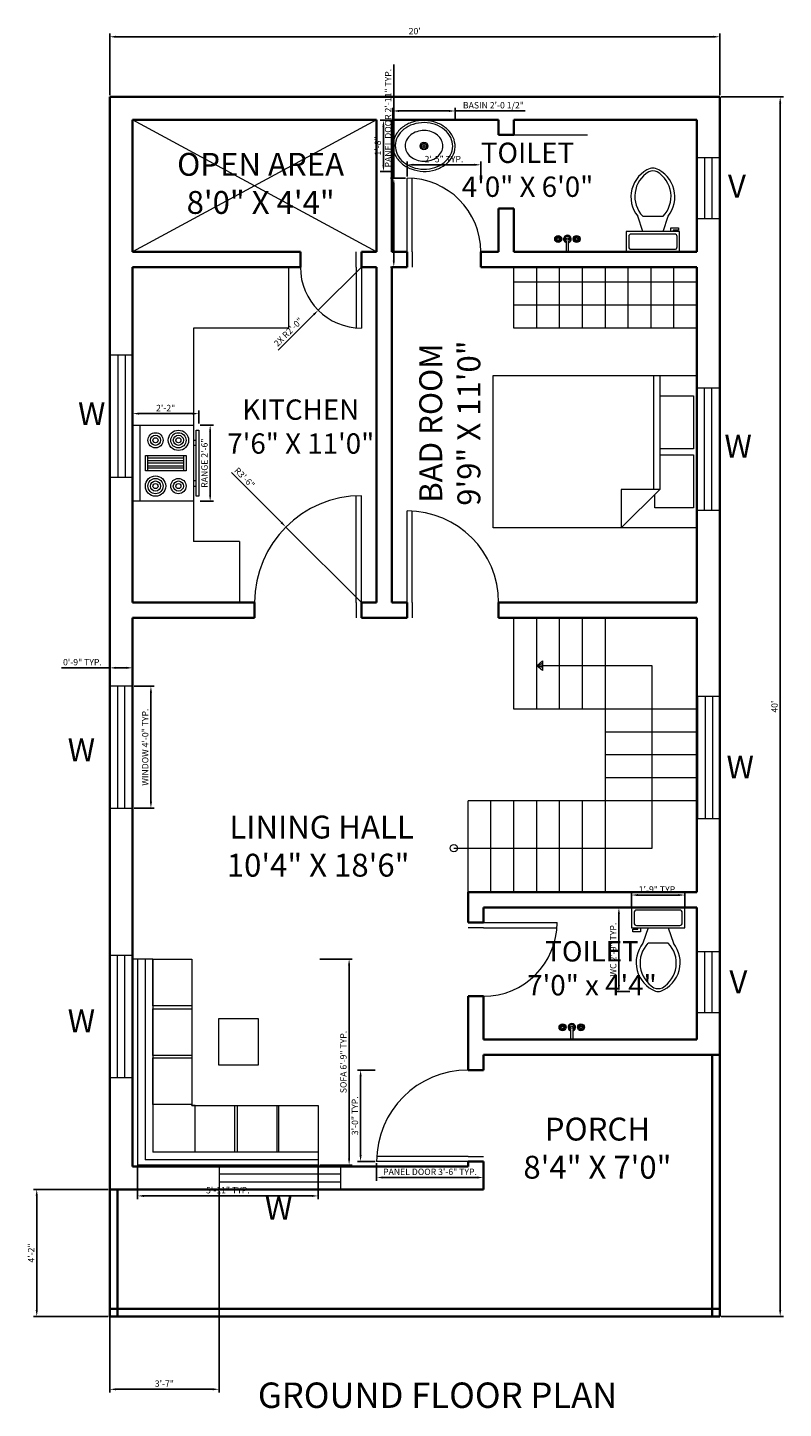
# Model space of a CAD drawing. Units: inches. Extents: x 1827 to 2455, y 1682 to 2281.
# Tile 1 of 3: x 1827 to 2124, y 1686 to 2229. Entities that reach past the tile are written whole.
import ezdxf

# ---------------------------------------------------------------- set-up
doc = ezdxf.new("R2010")
doc.units = ezdxf.units.IN
for name, color, linetype, lineweight in [('A-ANNO-DIMS', 2, 'Continuous', 18), ('A-ANNO-TEXT', 7, 'Continuous', 18), ('A-AREA-IDEN', 7, 'Continuous', 18), ('A-DOOR', 3, 'Continuous', 18), ('A-EQPM', 9, 'Continuous', 18), ('A-FLOR-CABN', 9, 'Continuous', 18), ('A-FLOR-FIXT', 9, 'Continuous', 18), ('A-FLOR-OPEN', 8, 'Continuous', 13), ('A-FLOR-STRS', 7, 'Continuous', 20), ('A-FURN', 8, 'Continuous', 18), ('A-GLAZ', 4, 'Continuous', 18), ('A-WALL', 7, 'Continuous', 35)]:
    doc.layers.add(name, color=color, linetype=linetype, lineweight=lineweight)
doc.styles.get("Standard").update_dxf_attribs({"font": 'arial.ttf'})
doc.dimstyles.new('ISO-25', dxfattribs={"dimtxt": 2.5, "dimasz": 2.5, "dimexe": 1.25, "dimexo": 0.625, "dimtad": 1, "dimdec": 0, "dimlunit": 3, "dimtxsty": 'Standard', "dimcen": 2.5, "dimadec": 0, "dimazin": 0, "dimtfac": 1, "dimtdec": 0, "dimtmove": 0, "dimatfit": 3, "dimfxl": 1, "dimarcsym": 0})

# ---------------------------------------------------------------- blocks, each defined once
blk = doc.blocks.new('Range-Oven - 30 in top')
for p, q in [((0, -3), (30, -3)), ((12, -6), (18, -6)), ((13, -20), (13, -6)), ((14, -6), (14, -20)), ((15, -20), (15, -6)), ((16, -6), (16, -20)), ((17, -20), (17, -6)), ((18, -20), (12, -20)), ((6, -24), (6, -25)), ((8, -25), (8, -24)), ((22, -25), (22, -24)), ((24, -24), (24, -25))]:
    blk.add_line(p, q)
for points in [[(0, -24), (0, 0), (30, 0), (30, -24)], [(12, -21), (12, -5), (18, -5), (18, -21)], [(2, -26), (2, -25), (28, -25), (28, -26)]]:
    blk.add_lwpolyline(points, close=True)
for centre, radius in [((6, -9), 4), ((6, -9), 3), ((6, -9), 2), ((6, -9), 1), ((24, -9), 3), ((24, -9), 2), ((24, -9), 1), ((6, -18), 3), ((6, -18), 2), ((24, -18), 4), ((24, -18), 3), ((24, -18), 2), ((6, -18), 1), ((24, -18), 1)]:
    blk.add_circle(centre, radius)
blk = doc.blocks.new('Bed - Queen')
for p, q in [((0, -80.00003), (0, 0)), ((0, 0), (59.99999, 0)), ((59.99999, 0), (59.99999, -80.00003)), ((7.99999, -1.2), (28.79998, -1.2)), ((7.99999, -14.4), (7.99999, -1.2)), ((28.79998, -1.2), (28.79998, -14.4)), ((31.19999, -1.2), (51.99999, -1.2)), ((31.19999, -14.4), (31.19999, -1.2)), ((51.99999, -1.2), (51.99999, -16.4)), ((0, -14.4), (44.8, -14.4)), ((59.99999, -29.6), (44.8, -14.4)), ((44.8, -14.4), (44.8, -29.6)), ((44.8, -16.8), (0, -16.8)), ((51.99999, -16.4), (46.79936, -16.4)), ((44.8, -29.6), (59.99999, -29.6)), ((59.99999, -80.00003), (0, -80.00003))]:
    blk.add_line(p, q)
blk = doc.blocks.new('Sink - Oval top')
for p, q in [((-1, 0), (1, 0)), ((0, 1), (0, -1))]:
    blk.add_line(p, q)
for points in [[(-12.23, 0.39, 0.117634), (-11.46, -3.36, 0.104469), (-8.88, -6.8, 0.090016), (-5.08, -9.07, 0.08192), (-0.32, -10.02, 0.08192), (4.49, -9.38, 0.090016), (8.42, -7.36, 0.104469), (11.22, -4.09, 0.117634), (12.23, -0.39, 0.117634), (11.46, 3.36, 0.104469), (8.88, 6.8, 0.090016), (5.08, 9.07, 0.08192), (0.32, 10.02, 0.08192), (-4.49, 9.38, 0.090016), (-8.42, 7.36, 0.104469), (-11.22, 4.09, 0.117634)], [(-11.29, 0.16, 0.118622), (-10.52, -3.25, 0.104678), (-8.07, -6.36, 0.089562), (-4.54, -8.37, 0.081185), (-0.13, -9.15, 0.081185), (4.3, -8.49, 0.089562), (7.89, -6.58, 0.104678), (10.42, -3.55, 0.118622), (11.29, -0.16, 0.118622), (10.52, 3.25, 0.104678), (8.07, 6.36, 0.089562), (4.54, 8.37, 0.081185), (0.13, 9.15, 0.081185), (-4.3, 8.49, 0.089562), (-7.89, 6.58, 0.104678), (-10.42, 3.55, 0.118622)], [(-7.42, 0.08, 0.118283), (-6.91, -2.17, 0.104607), (-5.29, -4.21, 0.089718), (-2.97, -5.53, 0.081436), (-0.07, -6.04, 0.081436), (2.84, -5.59, 0.089718), (5.2, -4.33, 0.104607), (6.86, -2.32, 0.118283), (7.42, -0.08, 0.118283), (6.91, 2.17, 0.104607), (5.29, 4.21, 0.089718), (2.97, 5.53, 0.081436), (0.07, 6.04, 0.081436), (-2.84, 5.59, 0.089718), (-5.2, 4.33, 0.104607), (-6.86, 2.32, 0.118283)]]:
    blk.add_lwpolyline(points, format="xyb", close=True)
for radius in [1.5, 1]:
    blk.add_circle((0, 0), radius)
blk = doc.blocks.new('Toilet - top')
for p, q in [((9.5, -6), (9.5, -2)), ((-10, -8.5), (-8, -8.5)), ((-10, -9.5), (-10, -8.5)), ((-7, -9.5), (-10, -9.5)), ((-8, -8.5), (-8, -8)), ((-7, -8), (-7, -9.5)), ((-4, -8), (-6, -14)), ((4, -8), (6, -14)), ((4, -14), (-4, -14))]:
    blk.add_line(p, q)
blk.add_lwpolyline([(10.5, -8), (10.5, 0), (-10.5, 0), (-10.5, -8)], close=True)
for points in [[(-9.5, -2), (-9.5, -6)], [(8.5, -1), (-8.5, -1)], [(-8.5, -7), (8.5, -7)]]:
    blk.add_lwpolyline(points)
for centre, radius, start, end in [((-8.62, -1.88), 0.884, 81.8699, 188.1301), ((8.62, -1.88), 0.884, 351.8699, 98.1301), ((-8.62, -6.12), 0.884, 171.8699, 278.1301), ((8.62, -6.12), 0.884, 261.8699, 8.1301), ((3.52, -21.58), 12.17, 141.4691, 247.9714), ((4.2, -21.82), 11.33, 136.3677, 238.9468), ((-3.52, -21.58), 12.17, 292.0284, 38.5307), ((-4.2, -21.82), 11.33, 301.053, 43.6321), ((0, -27.88), 4, 245.7318, 294.2682), ((0, -29), 4, 254.8605, 285.1395)]:
    blk.add_arc(centre, radius, start, end)
blk = doc.blocks.new('Faucet - Bathroom top')
for p, q in [((-4.107, 0.125), (-4.375, 0.125)), ((-3.75, 0.4788), (-3.75, 0.75)), ((-3.5, 0.482), (-3.5, 0.75)), ((-3.1461, 0.125), (-2.875, 0.125)), ((3.143, 0.125), (2.875, 0.125)), ((3.5, 0.4788), (3.5, 0.75)), ((3.75, 0.482), (3.75, 0.75)), ((4.1039, 0.125), (4.375, 0.125)), ((-4.1039, -0.125), (-4.375, -0.125)), ((-3.75, -0.4821), (-3.75, -0.75)), ((-3.5, -0.4789), (-3.5, -0.75)), ((-3.143, -0.125), (-2.875, -0.125)), ((-0.5, -0.8639), (-0.5, -4.5)), ((0.5, -4.5), (0.5, -0.8631)), ((3.1461, -0.125), (2.875, -0.125)), ((3.5, -0.4821), (3.5, -0.75)), ((3.75, -0.4789), (3.75, -0.75)), ((4.107, -0.125), (4.375, -0.125))]:
    blk.add_line(p, q)
for centre, radius in [((-3.625, 0), 1.375), ((-4.625, 0), 0.2795), ((-3.625, 0), 0.5), ((-3.625, 1), 0.2795), ((-2.625, 0), 0.2795), ((0, 0), 0.5), ((3.625, 0), 1.375), ((2.625, 0), 0.2795), ((3.625, 0), 0.5), ((3.625, 1), 0.2795), ((4.625, 0), 0.2795), ((-3.625, -1), 0.2795), ((3.625, -1), 0.2795)]:
    blk.add_circle(centre, radius)
for centre, radius, start, end in [((-3.625, 0), 1, 105.2407, 164.2093), ((-3.625, 0), 1, 16.44125, 74.07887), ((0, 0), 1.5, 289.6514, 250.3603), ((0, 0), 1, 300.3431, 239.7554), ((3.625, 0), 1, 106.12, 164.0884), ((3.625, 0), 1, 16.23422, 73.90469), ((-3.625, 0), 1, 196.2342, 253.9047), ((-3.625, 0), 1, 286.12, 344.0884), ((0, -4.5), 0.5, 180, 0), ((3.625, 0), 1, 196.4413, 254.0789), ((3.625, 0), 1, 285.2407, 344.2093)]:
    blk.add_arc(centre, radius, start, end)
blk = doc.blocks.new('*D11')
at = {"layer": 'A-ANNO-DIMS', "color": 0, "lineweight": -2, "transparency": 16777216}
for p, q in [((1859.1, 2202.38), (1859.1, 2226.63)), ((1861.6, 2225.38), (2096.6, 2225.38)), ((2099.1, 2202.38), (2099.1, 2226.63))]:
    blk.add_line(p, q, dxfattribs=at)
at = {"layer": 'A-ANNO-DIMS', "color": 0, "transparency": 16777216}
for points in [[(1861.6, 2225.79), (1861.6, 2224.96), (1859.1, 2225.38)], [(2096.6, 2225.79), (2096.6, 2224.96), (2099.1, 2225.38)]]:
    blk.add_solid(points, dxfattribs=at)
at = {"layer": 'Defpoints', "color": 0, "transparency": 16777216}
for p in [(2099.1, 2225.38), (1859.1, 2201.75), (2099.1, 2201.75)]:
    blk.add_point(p, dxfattribs=at)
at = {"layer": 'A-ANNO-DIMS', "color": 0, "transparency": 16777216, "insert": (1979.1, 2227.28), "char_height": 2.5, "attachment_point": 5}
blk.add_mtext("20'", dxfattribs=at)
blk = doc.blocks.new('*D12')
at = {"layer": 'A-ANNO-DIMS', "color": 0, "lineweight": -2, "transparency": 16777216}
for p, q in [((2099.72, 2201.75), (2124.15, 2201.75)), ((2122.9, 2199.25), (2122.9, 1724.25)), ((2099.72, 1721.75), (2124.15, 1721.75))]:
    blk.add_line(p, q, dxfattribs=at)
at = {"layer": 'A-ANNO-DIMS', "color": 0, "transparency": 16777216}
for points in [[(2122.48, 2199.25), (2123.32, 2199.25), (2122.9, 2201.75)], [(2122.48, 1724.25), (2123.32, 1724.25), (2122.9, 1721.75)]]:
    blk.add_solid(points, dxfattribs=at)
at = {"layer": 'Defpoints', "color": 0, "transparency": 16777216}
for p in [(2099.1, 2201.75), (2099.1, 1721.75), (2122.9, 1721.75)]:
    blk.add_point(p, dxfattribs=at)
at = {"layer": 'A-ANNO-DIMS', "color": 0, "transparency": 16777216, "insert": (2121, 1961.75), "char_height": 2.5, "attachment_point": 5, "rotation": 90}
blk.add_mtext("40'", dxfattribs=at)
blk = doc.blocks.new('WIN-48IN')
for p, q in [((48, 9), (0, 9)), ((0, 9), (0, 0)), ((48, 6), (0, 6)), ((48, 0), (48, 9)), ((0, 3), (48, 3)), ((0, 0), (48, 0))]:
    blk.add_line(p, q)
blk = doc.blocks.new('VENT-24IN')
for p, q in [((0, 24), (0, 0)), ((0, 24), (9, 24)), ((3, 24), (3, 0)), ((6, 0), (6, 24)), ((9, 0), (9, 24)), ((0, 0), (9, 0))]:
    blk.add_line(p, q)
blk = doc.blocks.new('DOOR-29IN-PANEL')
for p, q in [((0, 6), (0, 35)), ((2, 6), (2, 35)), ((2, 6), (2, 0))]:
    blk.add_line(p, q)
blk.add_arc((0, 6), 29, 0, 90)
blk = doc.blocks.new('DOOR-36IN-PANEL')
for p, q in [((0, 6), (0, 42)), ((2, 6), (2, 42)), ((2, 6), (2, 0))]:
    blk.add_line(p, q)
blk.add_arc((0, 6), 36, 0, 90)
blk = doc.blocks.new('SOFA-L-SECTIONAL')
for p, q in [((0, 81.06), (0, 23.78)), ((3, 81.06), (3, 23.78)), ((6, 81.06), (6, 23.78)), ((21.43, 81.06), (21.43, 23.78)), ((0, 23.78), (0, 5)), ((3, 23.78), (3, 5)), ((6, 23.78), (6, 5)), ((21.43, 23.38), (21.43, 23.78)), ((21.43, 23.78), (21.43, 23.38)), ((22.69, 23.38), (21.43, 23.38)), ((21.43, 23.38), (39.33, 23.38)), ((22.69, 5), (22.69, 23.38)), ((39.33, 23.38), (71.09, 23.38)), ((0, 5), (0, 0)), ((3, 5), (3, 2)), ((6, 2), (3, 2)), ((22.69, 5), (6, 5)), ((22.69, 2), (6, 2)), ((71.09, 5), (22.69, 5)), ((71.09, 2), (22.69, 2)), ((71.09, 5), (71.09, 0)), ((6, 0), (0, 0)), ((22.69, 0), (6, 0)), ((71.09, 0), (22.69, 0))]:
    blk.add_line(p, q)
for points in [[(6, 81.06), (21.43, 81.06), (21.43, 62.67), (6, 62.67)], [(6, 61.41), (21.43, 61.41), (21.43, 43.03), (6, 43.03)], [(6, 42.16), (21.43, 42.16), (21.43, 23.78), (6, 23.78)], [(22.69, 23.38), (38.12, 23.38), (38.12, 5), (22.69, 5)], [(39.33, 23.38), (54.76, 23.38), (54.76, 5), (39.33, 5)], [(55.66, 23.38), (71.09, 23.38), (71.09, 5), (55.66, 5)]]:
    blk.add_lwpolyline(points, close=True)
blk = doc.blocks.new('TABLE-OCCASIONAL')
blk.add_lwpolyline([(0, 18.39), (15.43, 18.39), (15.43, 0), (0, 0)], close=True)
blk = doc.blocks.new('*D27')
at = {"layer": 'A-ANNO-DIMS', "color": 0, "lineweight": -2, "transparency": 16777216}
for p, q in [((1868.71, 1969.82), (1876.54, 1969.82)), ((1875.29, 1924.32), (1875.29, 1967.32)), ((1868.71, 1921.82), (1876.54, 1921.82))]:
    blk.add_line(p, q, dxfattribs=at)
at = {"layer": 'A-ANNO-DIMS', "color": 0, "transparency": 16777216}
for points in [[(1874.87, 1967.32), (1875.7, 1967.32), (1875.29, 1969.82)], [(1874.87, 1924.32), (1875.7, 1924.32), (1875.29, 1921.82)]]:
    blk.add_solid(points, dxfattribs=at)
at = {"layer": 'Defpoints', "color": 0, "transparency": 16777216}
for p in [(1868.09, 1969.82), (1875.29, 1969.82), (1868.09, 1921.82)]:
    blk.add_point(p, dxfattribs=at)
at = {"layer": 'A-ANNO-DIMS', "color": 0, "transparency": 16777216, "insert": (1873.37, 1945.82), "char_height": 2.5, "attachment_point": 5, "rotation": 90}
blk.add_mtext('WINDOW 4\'-0" TYP.', dxfattribs=at)
blk = doc.blocks.new('*D28')
at = {"layer": 'A-ANNO-DIMS', "color": 0, "lineweight": -2, "transparency": 16777216}
for p, q in [((1859.09, 1970.44), (1859.09, 1978.27)), ((1868.09, 1970.44), (1868.09, 1978.27)), ((1859.09, 1977.02), (1840.1, 1977.02)), ((1865.59, 1977.02), (1861.59, 1977.02))]:
    blk.add_line(p, q, dxfattribs=at)
at = {"layer": 'A-ANNO-DIMS', "color": 0, "transparency": 16777216}
for points in [[(1861.59, 1977.44), (1861.59, 1976.6), (1859.09, 1977.02)], [(1865.59, 1977.44), (1865.59, 1976.6), (1868.09, 1977.02)]]:
    blk.add_solid(points, dxfattribs=at)
at = {"layer": 'Defpoints', "color": 0, "transparency": 16777216}
for p in [(1859.09, 1977.02), (1859.09, 1969.82), (1868.09, 1969.82)]:
    blk.add_point(p, dxfattribs=at)
at = {"layer": 'A-ANNO-DIMS', "color": 0, "transparency": 16777216, "insert": (1848.34, 1978.92), "char_height": 2.5, "attachment_point": 5}
blk.add_mtext('0\'-9" TYP.', dxfattribs=at)
blk = doc.blocks.new('*D35')
at = {"layer": 'A-ANNO-DIMS', "color": 0, "lineweight": -2, "transparency": 16777216}
for p, q in [((2063.76, 1882.65), (2058.18, 1882.65)), ((2059.43, 1852.1), (2059.43, 1880.15)), ((2063.76, 1849.6), (2058.18, 1849.6))]:
    blk.add_line(p, q, dxfattribs=at)
at = {"layer": 'A-ANNO-DIMS', "color": 0, "transparency": 16777216}
for points in [[(2059.01, 1880.15), (2059.84, 1880.15), (2059.43, 1882.65)], [(2059.01, 1852.1), (2059.84, 1852.1), (2059.43, 1849.6)]]:
    blk.add_solid(points, dxfattribs=at)
at = {"layer": 'Defpoints', "color": 0, "transparency": 16777216}
for p in [(2059.43, 1882.65), (2064.38, 1882.65), (2064.38, 1849.6)]:
    blk.add_point(p, dxfattribs=at)
at = {"layer": 'A-ANNO-DIMS', "color": 0, "transparency": 16777216, "insert": (2057.51, 1866.13), "char_height": 2.5, "attachment_point": 5, "rotation": 90}
blk.add_mtext('WC 2\'-9" TYP.', dxfattribs=at)
blk = doc.blocks.new('*D36')
at = {"layer": 'A-ANNO-DIMS', "color": 0, "lineweight": -2, "transparency": 16777216}
for p, q in [((2064.38, 1883.27), (2064.38, 1888.86)), ((2066.88, 1887.61), (2082.88, 1887.61)), ((2085.38, 1883.27), (2085.38, 1888.86))]:
    blk.add_line(p, q, dxfattribs=at)
at = {"layer": 'A-ANNO-DIMS', "color": 0, "transparency": 16777216}
for points in [[(2066.88, 1888.02), (2066.88, 1887.19), (2064.38, 1887.61)], [(2082.88, 1888.02), (2082.88, 1887.19), (2085.38, 1887.61)]]:
    blk.add_solid(points, dxfattribs=at)
at = {"layer": 'Defpoints', "color": 0, "transparency": 16777216}
for p in [(2085.38, 1887.61), (2064.38, 1882.65), (2085.38, 1882.65)]:
    blk.add_point(p, dxfattribs=at)
at = {"layer": 'A-ANNO-DIMS', "color": 0, "transparency": 16777216, "insert": (2074.88, 1889.51), "char_height": 2.5, "attachment_point": 5}
blk.add_mtext('1\'-9" TYP.', dxfattribs=at)
blk = doc.blocks.new('*D37')
at = {"layer": 'A-ANNO-DIMS', "color": 0, "lineweight": -2, "transparency": 16777216}
for p, q in [((1970.85, 2169.75), (1970.85, 2214.43)), ((1975.47, 2169.75), (1969.6, 2169.75)), ((1970.85, 2137.25), (1970.85, 2167.25)), ((1975.47, 2134.75), (1969.6, 2134.75))]:
    blk.add_line(p, q, dxfattribs=at)
at = {"layer": 'A-ANNO-DIMS', "color": 0, "transparency": 16777216}
for points in [[(1970.43, 2167.25), (1971.26, 2167.25), (1970.85, 2169.75)], [(1970.43, 2137.25), (1971.26, 2137.25), (1970.85, 2134.75)]]:
    blk.add_solid(points, dxfattribs=at)
at = {"layer": 'Defpoints', "color": 0, "transparency": 16777216}
for p in [(1970.85, 2169.75), (1976.1, 2169.75), (1976.1, 2134.75)]:
    blk.add_point(p, dxfattribs=at)
at = {"layer": 'A-ANNO-DIMS', "color": 0, "transparency": 16777216, "insert": (1968.93, 2193.34), "char_height": 2.5, "attachment_point": 5, "rotation": 90}
blk.add_mtext('PANEL DOOR 2\'-11" TYP.', dxfattribs=at)
blk = doc.blocks.new('*D38')
at = {"layer": 'A-ANNO-DIMS', "color": 0, "lineweight": -2, "transparency": 16777216}
for p, q in [((1976.1, 2170.38), (1976.1, 2176.25)), ((1978.6, 2175), (2002.6, 2175)), ((2005.1, 2170.38), (2005.1, 2176.25))]:
    blk.add_line(p, q, dxfattribs=at)
at = {"layer": 'A-ANNO-DIMS', "color": 0, "transparency": 16777216}
for points in [[(1978.6, 2175.42), (1978.6, 2174.59), (1976.1, 2175)], [(2002.6, 2175.42), (2002.6, 2174.59), (2005.1, 2175)]]:
    blk.add_solid(points, dxfattribs=at)
at = {"layer": 'Defpoints', "color": 0, "transparency": 16777216}
for p in [(2005.1, 2175), (1976.1, 2169.75), (2005.1, 2169.75)]:
    blk.add_point(p, dxfattribs=at)
at = {"layer": 'A-ANNO-DIMS', "color": 0, "transparency": 16777216, "insert": (1990.6, 2176.91), "char_height": 2.5, "attachment_point": 5}
blk.add_mtext('2\'-5" TYP.', dxfattribs=at)
blk = doc.blocks.new('*D39')
at = {"layer": 'A-ANNO-DIMS', "color": 0, "lineweight": -2, "transparency": 16777216}
for p, q in [((1964.1, 1782.13), (1964.1, 1775.2)), ((2006.1, 1782.13), (2006.1, 1775.2)), ((2003.6, 1776.45), (1966.6, 1776.45))]:
    blk.add_line(p, q, dxfattribs=at)
at = {"layer": 'A-ANNO-DIMS', "color": 0, "transparency": 16777216}
for points in [[(1966.6, 1776.87), (1966.6, 1776.04), (1964.1, 1776.45)], [(2003.6, 1776.87), (2003.6, 1776.04), (2006.1, 1776.45)]]:
    blk.add_solid(points, dxfattribs=at)
at = {"layer": 'Defpoints', "color": 0, "transparency": 16777216}
for p in [(1964.1, 1782.75), (2006.1, 1782.75), (1964.1, 1776.45)]:
    blk.add_point(p, dxfattribs=at)
at = {"layer": 'A-ANNO-DIMS', "color": 0, "transparency": 16777216, "insert": (1985.1, 1778.37), "char_height": 2.5, "attachment_point": 5}
blk.add_mtext('PANEL DOOR 3\'-6" TYP.', dxfattribs=at)
blk = doc.blocks.new('*D40')
at = {"layer": 'A-ANNO-DIMS', "color": 0, "lineweight": -2, "transparency": 16777216}
for p, q in [((1963.47, 1818.75), (1956.55, 1818.75)), ((1957.8, 1785.25), (1957.8, 1816.25)), ((1963.47, 1782.75), (1956.55, 1782.75))]:
    blk.add_line(p, q, dxfattribs=at)
at = {"layer": 'A-ANNO-DIMS', "color": 0, "transparency": 16777216}
for points in [[(1957.38, 1816.25), (1958.21, 1816.25), (1957.8, 1818.75)], [(1957.38, 1785.25), (1958.21, 1785.25), (1957.8, 1782.75)]]:
    blk.add_solid(points, dxfattribs=at)
at = {"layer": 'Defpoints', "color": 0, "transparency": 16777216}
for p in [(1957.8, 1818.75), (1964.1, 1818.75), (1964.1, 1782.75)]:
    blk.add_point(p, dxfattribs=at)
at = {"layer": 'A-ANNO-DIMS', "color": 0, "transparency": 16777216, "insert": (1955.89, 1800.75), "char_height": 2.5, "attachment_point": 5, "rotation": 90}
blk.add_mtext('3\'-0" TYP.', dxfattribs=at)
blk = doc.blocks.new('*D45')
at = {"layer": 'A-ANNO-DIMS', "color": 0, "lineweight": -2, "transparency": 16777216}
for p, q in [((1941.73, 1862.43), (1954.52, 1862.43)), ((1953.27, 1783.87), (1953.27, 1859.93)), ((1941.73, 1781.37), (1954.52, 1781.37))]:
    blk.add_line(p, q, dxfattribs=at)
at = {"layer": 'A-ANNO-DIMS', "color": 0, "transparency": 16777216}
for points in [[(1952.85, 1859.93), (1953.68, 1859.93), (1953.27, 1862.43)], [(1952.85, 1783.87), (1953.68, 1783.87), (1953.27, 1781.37)]]:
    blk.add_solid(points, dxfattribs=at)
at = {"layer": 'Defpoints', "color": 0, "transparency": 16777216}
for p in [(1941.11, 1862.43), (1953.27, 1862.43), (1941.11, 1781.37)]:
    blk.add_point(p, dxfattribs=at)
at = {"layer": 'A-ANNO-DIMS', "color": 0, "transparency": 16777216, "insert": (1951.35, 1821.9), "char_height": 2.5, "attachment_point": 5, "rotation": 90}
blk.add_mtext('SOFA 6\'-9" TYP.', dxfattribs=at)
blk = doc.blocks.new('*D46')
at = {"layer": 'A-ANNO-DIMS', "color": 0, "lineweight": -2, "transparency": 16777216}
for p, q in [((1870.02, 1780.74), (1870.02, 1767.96)), ((1941.11, 1780.74), (1941.11, 1767.96)), ((1872.52, 1769.21), (1938.61, 1769.21))]:
    blk.add_line(p, q, dxfattribs=at)
at = {"layer": 'A-ANNO-DIMS', "color": 0, "transparency": 16777216}
for points in [[(1872.52, 1769.63), (1872.52, 1768.79), (1870.02, 1769.21)], [(1938.61, 1769.63), (1938.61, 1768.79), (1941.11, 1769.21)]]:
    blk.add_solid(points, dxfattribs=at)
at = {"layer": 'Defpoints', "color": 0, "transparency": 16777216}
for p in [(1870.02, 1781.37), (1941.11, 1781.37), (1941.11, 1769.21)]:
    blk.add_point(p, dxfattribs=at)
at = {"layer": 'A-ANNO-DIMS', "color": 0, "transparency": 16777216, "insert": (1905.56, 1771.11), "char_height": 2.5, "attachment_point": 5}
blk.add_mtext('5\'-11" TYP.', dxfattribs=at)
blk = doc.blocks.new('*D49')
at = {"layer": 'A-ANNO-DIMS', "color": 0, "lineweight": -2, "transparency": 16777216}
for p, q in [((1970.47, 2193.13), (1970.47, 2197.43)), ((1972.97, 2196.18), (1992.52, 2196.18)), ((1995.02, 2193.13), (1995.02, 2197.43)), ((1995.02, 2196.18), (2022.58, 2196.18))]:
    blk.add_line(p, q, dxfattribs=at)
at = {"layer": 'A-ANNO-DIMS', "color": 0, "transparency": 16777216}
for points in [[(1972.97, 2196.6), (1972.97, 2195.77), (1970.47, 2196.18)], [(1992.52, 2196.6), (1992.52, 2195.77), (1995.02, 2196.18)]]:
    blk.add_solid(points, dxfattribs=at)
at = {"layer": 'Defpoints', "color": 0, "transparency": 16777216}
for p in [(1995.02, 2196.18), (1970.47, 2192.5), (1995.02, 2192.5)]:
    blk.add_point(p, dxfattribs=at)
at = {"layer": 'A-ANNO-DIMS', "color": 0, "transparency": 16777216, "insert": (2010.05, 2198.1), "char_height": 2.5, "attachment_point": 5}
blk.add_mtext('BASIN 2\'-0 1/2"', dxfattribs=at)
blk = doc.blocks.new('*D50')
at = {"layer": 'A-ANNO-DIMS', "color": 0, "lineweight": -2, "transparency": 16777216}
for p, q in [((1969.84, 2192.5), (1965.54, 2192.5)), ((1966.79, 2174.86), (1966.79, 2190)), ((1969.84, 2172.36), (1965.54, 2172.36))]:
    blk.add_line(p, q, dxfattribs=at)
at = {"layer": 'A-ANNO-DIMS', "color": 0, "transparency": 16777216}
for points in [[(1966.37, 2190), (1967.2, 2190), (1966.79, 2192.5)], [(1966.37, 2174.86), (1967.2, 2174.86), (1966.79, 2172.36)]]:
    blk.add_solid(points, dxfattribs=at)
at = {"layer": 'Defpoints', "color": 0, "transparency": 16777216}
for p in [(1966.79, 2192.5), (1970.47, 2192.5), (1970.47, 2172.36)]:
    blk.add_point(p, dxfattribs=at)
at = {"layer": 'A-ANNO-DIMS', "color": 0, "transparency": 16777216, "insert": (1964.88, 2182.43), "char_height": 2.5, "attachment_point": 5, "rotation": 90}
blk.add_mtext('1\'-8"', dxfattribs=at)
blk = doc.blocks.new('*D51')
at = {"layer": 'A-ANNO-DIMS', "color": 0, "lineweight": -2, "transparency": 16777216}
for p, q in [((1894.72, 2072.57), (1899.85, 2072.57)), ((1898.6, 2045.07), (1898.6, 2070.07)), ((1894.72, 2042.57), (1899.85, 2042.57))]:
    blk.add_line(p, q, dxfattribs=at)
at = {"layer": 'A-ANNO-DIMS', "color": 0, "transparency": 16777216}
for points in [[(1898.18, 2070.07), (1899.01, 2070.07), (1898.6, 2072.57)], [(1898.18, 2045.07), (1899.01, 2045.07), (1898.6, 2042.57)]]:
    blk.add_solid(points, dxfattribs=at)
at = {"layer": 'Defpoints', "color": 0, "transparency": 16777216}
for p in [(1894.1, 2072.57), (1898.6, 2072.57), (1894.1, 2042.57)]:
    blk.add_point(p, dxfattribs=at)
at = {"layer": 'A-ANNO-DIMS', "color": 0, "transparency": 16777216, "insert": (1896.68, 2057.57), "char_height": 2.5, "attachment_point": 5, "rotation": 90}
blk.add_mtext('RANGE 2\'-6"', dxfattribs=at)
blk = doc.blocks.new('*D52')
at = {"layer": 'A-ANNO-DIMS', "color": 0, "lineweight": -2, "transparency": 16777216}
for p, q in [((1868.1, 2073.19), (1868.1, 2078.32)), ((1891.6, 2077.07), (1870.6, 2077.07)), ((1894.1, 2073.19), (1894.1, 2078.32))]:
    blk.add_line(p, q, dxfattribs=at)
at = {"layer": 'A-ANNO-DIMS', "color": 0, "transparency": 16777216}
for points in [[(1870.6, 2077.48), (1870.6, 2076.65), (1868.1, 2077.07)], [(1891.6, 2077.48), (1891.6, 2076.65), (1894.1, 2077.07)]]:
    blk.add_solid(points, dxfattribs=at)
at = {"layer": 'Defpoints', "color": 0, "transparency": 16777216}
for p in [(1868.1, 2077.07), (1868.1, 2072.57), (1894.1, 2072.57)]:
    blk.add_point(p, dxfattribs=at)
at = {"layer": 'A-ANNO-DIMS', "color": 0, "transparency": 16777216, "insert": (1881.1, 2078.95), "char_height": 2.5, "attachment_point": 5}
blk.add_mtext('2\'-2"', dxfattribs=at)
blk = doc.blocks.new('*D57')
at = {"layer": 'A-ANNO-DIMS', "color": 0, "lineweight": -2, "transparency": 16777216}
for p, q in [((1858.47, 1771.75), (1829.11, 1771.75)), ((1830.36, 1724.25), (1830.36, 1769.25)), ((1858.47, 1721.75), (1829.11, 1721.75))]:
    blk.add_line(p, q, dxfattribs=at)
at = {"layer": 'A-ANNO-DIMS', "color": 0, "transparency": 16777216}
for points in [[(1829.94, 1769.25), (1830.78, 1769.25), (1830.36, 1771.75)], [(1829.94, 1724.25), (1830.78, 1724.25), (1830.36, 1721.75)]]:
    blk.add_solid(points, dxfattribs=at)
at = {"layer": 'Defpoints', "color": 0, "transparency": 16777216}
for p in [(1830.36, 1771.75), (1859.1, 1771.75), (1859.1, 1721.75)]:
    blk.add_point(p, dxfattribs=at)
at = {"layer": 'A-ANNO-DIMS', "color": 0, "transparency": 16777216, "insert": (1828.48, 1746.75), "char_height": 2.5, "attachment_point": 5, "rotation": 90}
blk.add_mtext('4\'-2"', dxfattribs=at)
blk = doc.blocks.new('*D59')
at = {"layer": 'A-ANNO-DIMS', "color": 0, "lineweight": -2, "transparency": 16777216}
for p, q in [((1859.1, 1771.13), (1859.1, 1691.85)), ((1902.08, 1771.13), (1902.08, 1691.85)), ((1861.6, 1693.1), (1899.58, 1693.1))]:
    blk.add_line(p, q, dxfattribs=at)
at = {"layer": 'A-ANNO-DIMS', "color": 0, "transparency": 16777216}
for points in [[(1861.6, 1693.52), (1861.6, 1692.69), (1859.1, 1693.1)], [(1899.58, 1693.52), (1899.58, 1692.69), (1902.08, 1693.1)]]:
    blk.add_solid(points, dxfattribs=at)
at = {"layer": 'Defpoints', "color": 0, "transparency": 16777216}
for p in [(1859.1, 1771.75), (1902.08, 1771.75), (1902.08, 1693.1)]:
    blk.add_point(p, dxfattribs=at)
at = {"layer": 'A-ANNO-DIMS', "color": 0, "transparency": 16777216, "insert": (1880.59, 1695.01), "char_height": 2.5, "attachment_point": 5}
blk.add_mtext('3\'-7"', dxfattribs=at)
blk = doc.blocks.new('*D62')
at = {"layer": 'A-ANNO-DIMS', "color": 0, "lineweight": -2, "transparency": 16777216}
for p, q in [((1906.94, 2053.91), (1926.63, 2034.22)), ((1958.1, 2002.75), (1928.4, 2032.45))]:
    blk.add_line(p, q, dxfattribs=at)
at = {"layer": 'A-ANNO-DIMS', "color": 0, "transparency": 16777216}
blk.add_solid([(1926.92, 2034.51), (1926.33, 2033.93), (1928.4, 2032.45)], dxfattribs=at)
at = {"layer": 'Defpoints', "color": 0, "transparency": 16777216}
for p in [(1928.4, 2032.45), (1958.1, 2002.75)]:
    blk.add_point(p, dxfattribs=at)
at = {"layer": 'A-ANNO-DIMS', "color": 0, "transparency": 16777216, "insert": (1911.92, 2051.62), "char_height": 2.5, "attachment_point": 5, "rotation": 315.0002}
blk.add_mtext('R3\'-6"', dxfattribs=at)
blk = doc.blocks.new('*D63')
at = {"layer": 'A-ANNO-DIMS', "color": 0, "lineweight": -2, "transparency": 16777216}
for p, q in [((1958.1, 2134.75), (1941.13, 2117.78)), ((1925.39, 2102.05), (1939.36, 2116.02))]:
    blk.add_line(p, q, dxfattribs=at)
at = {"layer": 'A-ANNO-DIMS', "color": 0, "transparency": 16777216}
blk.add_solid([(1939.06, 2116.31), (1939.65, 2115.72), (1941.13, 2117.78)], dxfattribs=at)
at = {"layer": 'Defpoints', "color": 0, "transparency": 16777216}
for p in [(1958.1, 2134.75), (1941.13, 2117.78)]:
    blk.add_point(p, dxfattribs=at)
at = {"layer": 'A-ANNO-DIMS', "color": 0, "transparency": 16777216, "insert": (1929.6, 2108.95), "char_height": 2.5, "attachment_point": 5, "rotation": 45.0007}
blk.add_mtext('2X R2\'-0"', dxfattribs=at)

msp = doc.modelspace()

# ---------------------------------------------------------------- linework, layer by layer
at = {"layer": 'A-DOOR'}
for p, q in [((2018.1, 2186.75), (2047.1, 2186.75)), ((1956.1, 2134.75), (1956.1, 2140.75)), ((1956.1, 2134.75), (1956.1, 2110.75)), ((1958.1, 2134.75), (1958.1, 2110.75)), ((1956.1, 2002.75), (1956.1, 2044.75)), ((1958.1, 2002.75), (1958.1, 2044.75)), ((1956.1, 2002.75), (1956.1, 1996.75))]:
    msp.add_line(p, q, dxfattribs=at)
for centre, radius, start, end in [((1958.1, 2134.75), 24, 180, 270), ((1958.1, 2002.75), 42, 90, 180)]:
    msp.add_arc(centre, radius, start, end, dxfattribs=at)
at = {"layer": 'A-FLOR-CABN'}
for p, q in [((1929.43, 2134.75), (1929.43, 2110.75)), ((2018.1, 2110.75), (2018.1, 2134.75)), ((2027.1, 2110.75), (2027.1, 2134.75)), ((2036.1, 2110.75), (2036.1, 2134.75)), ((2045.1, 2110.75), (2045.1, 2134.75)), ((2054.1, 2110.75), (2054.1, 2134.75)), ((2063.1, 2110.75), (2063.1, 2134.75)), ((2072.1, 2110.75), (2072.1, 2134.75)), ((2081.1, 2110.75), (2081.1, 2134.75)), ((2090.1, 2134.75), (2090.1, 2110.75)), ((2090.1, 2128.75), (2018.1, 2128.75)), ((2090.1, 2119.75), (2018.1, 2119.75)), ((1892.1, 2110.75), (1892.1, 2026.75)), ((1929.43, 2110.75), (1892.1, 2110.75)), ((2090.1, 2110.75), (2018.1, 2110.75)), ((1910.21, 2026.75), (1892.1, 2026.75)), ((1910.21, 2026.75), (1910.21, 2002.75))]:
    msp.add_line(p, q, dxfattribs=at)
at = {"layer": 'A-FLOR-OPEN'}
for p, q in [((1964.1, 2140.75), (1868.1, 2192.75)), ((1868.1, 2192.75), (1964.1, 2192.75)), ((1964.1, 2192.75), (1868.1, 2140.75))]:
    msp.add_line(p, q, dxfattribs=at)
at = {"layer": 'A-FLOR-STRS'}
for p, q in [((2018.1, 1960.75), (2018.1, 1996.75)), ((2027.1, 1960.75), (2027.1, 1996.75)), ((2036.1, 1960.75), (2036.1, 1996.75)), ((2045.1, 1960.75), (2045.1, 1996.75)), ((2054.1, 1888.75), (2054.1, 1996.75)), ((2029.41, 1979.79), (2027.1, 1977.86)), ((2027.1, 1977.86), (2029.41, 1978.81)), ((2029.41, 1977.82), (2029.41, 1979.79)), ((2029.41, 1979.79), (2029.41, 1975.98)), ((2029.41, 1977.88), (2029.41, 1979.79)), ((2029.41, 1978.81), (2029.41, 1977.12)), ((2027.1, 1977.86), (2029.41, 1977.88)), ((2029.41, 1975.98), (2027.1, 1977.86)), ((2029.41, 1977.12), (2027.13, 1977.87)), ((2072.51, 1977.82), (2029.41, 1977.82)), ((2072.51, 1906.05), (2072.51, 1977.82)), ((2090.1, 1960.75), (2018.1, 1960.75)), ((2090.1, 1951.75), (2054.1, 1951.75)), ((2090.1, 1942.75), (2054.1, 1942.75)), ((2090.1, 1933.75), (2054.1, 1933.75)), ((2000.1, 1888.75), (2000.1, 1924.75)), ((2009.1, 1924.75), (2000.1, 1924.75)), ((2090.1, 1924.75), (2009.1, 1924.75)), ((2009.1, 1888.75), (2009.1, 1924.75)), ((2018.1, 1888.75), (2018.1, 1924.75)), ((2027.1, 1888.75), (2027.1, 1924.75)), ((2036.1, 1888.75), (2036.1, 1924.75)), ((2045.1, 1888.75), (2045.1, 1924.75)), ((1994.51, 1906.05), (2072.51, 1906.05))]:
    msp.add_line(p, q, dxfattribs=at)
msp.add_circle((1994.51, 1906.05), 1.46, dxfattribs=at)
at = {"layer": 'A-FURN'}
msp.add_line((1876.02, 1862.43), (1868.1, 1862.43), dxfattribs=at)
at = {"layer": 'A-WALL'}
for p, q in [((1859.1, 2201.75), (1859.1, 1721.75)), ((2099.1, 2201.75), (1859.1, 2201.75)), ((2099.1, 1721.75), (2099.1, 2201.75)), ((1868.1, 2192.75), (1868.1, 2140.75)), ((1964.1, 2192.75), (1868.1, 2192.75)), ((1964.1, 2192.75), (1964.1, 2140.75)), ((1970.1, 2192.75), (1970.1, 2140.75)), ((2012.1, 2192.75), (1970.1, 2192.75)), ((2012.1, 2192.75), (2012.1, 2186.75)), ((2012.1, 2186.75), (2012.1, 2192.75)), ((2090.1, 2192.75), (2018.1, 2192.75)), ((2018.1, 2186.75), (2018.1, 2192.75)), ((2090.1, 2140.75), (2090.1, 2192.75)), ((2012.1, 2186.75), (2018.1, 2186.75)), ((2012.1, 2186.75), (2018.1, 2186.75)), ((2012.1, 2140.75), (2012.1, 2157.75)), ((2018.1, 2157.75), (2012.1, 2157.75)), ((2018.1, 2140.75), (2018.1, 2157.75)), ((1934.1, 2140.75), (1868.1, 2140.75)), ((1934.1, 2140.75), (1934.1, 2134.75)), ((1964.1, 2140.75), (1958.1, 2140.75)), ((1958.1, 2134.75), (1958.1, 2140.75)), ((1970.1, 2140.75), (1976.1, 2140.75)), ((1976.1, 2140.75), (1970.1, 2140.75)), ((1976.1, 2140.75), (1976.1, 2134.75)), ((2012.1, 2140.75), (2005.1, 2140.75)), ((2005.1, 2134.75), (2005.1, 2140.75)), ((2090.1, 2140.75), (2018.1, 2140.75)), ((1868.1, 2134.75), (1868.1, 2002.75)), ((1934.1, 2134.75), (1868.1, 2134.75)), ((1964.1, 2134.75), (1958.1, 2134.75)), ((1964.1, 2134.75), (1958.1, 2134.75)), ((1964.1, 2134.75), (1964.1, 2002.75)), ((1970.1, 2134.75), (1970.1, 2002.75)), ((1976.1, 2134.75), (1970.1, 2134.75)), ((2090.1, 2134.75), (2005.1, 2134.75)), ((2090.1, 2002.75), (2090.1, 2134.75)), ((1916.1, 2002.75), (1868.1, 2002.75)), ((1916.1, 1996.75), (1916.1, 2002.75)), ((1964.1, 2002.75), (1958.1, 2002.75)), ((1964.1, 2002.75), (1958.1, 2002.75)), ((1958.1, 2002.75), (1958.1, 1996.75)), ((1970.1, 2002.75), (1976.1, 2002.75)), ((1976.1, 2002.75), (1970.1, 2002.75)), ((1976.1, 2002.75), (1976.1, 1996.75)), ((2090.1, 2002.75), (2012.1, 2002.75)), ((2012.1, 1996.75), (2012.1, 2002.75)), ((1868.1, 1996.75), (1868.1, 1780.75)), ((1916.1, 1996.75), (1868.1, 1996.75)), ((1976.1, 1996.75), (1958.1, 1996.75)), ((2090.1, 1996.75), (2012.1, 1996.75)), ((2090.1, 1888.75), (2090.1, 1996.75)), ((2006.1, 1888.75), (2000.1, 1888.75)), ((2000.1, 1876.75), (2000.1, 1888.75)), ((2090.1, 1888.75), (2006.1, 1888.75)), ((2090.1, 1882.75), (2006.1, 1882.75)), ((2006.1, 1882.75), (2006.1, 1876.75)), ((2006.1, 1876.75), (2006.1, 1882.75)), ((2090.1, 1872.75), (2090.1, 1882.75)), ((2006.1, 1876.75), (2000.1, 1876.75)), ((2090.1, 1872.75), (2090.1, 1866.75)), ((2090.1, 1830.75), (2090.1, 1866.75)), ((2000.1, 1847.75), (2006.1, 1847.75)), ((2000.1, 1818.75), (2000.1, 1847.75)), ((2006.1, 1830.75), (2006.1, 1847.75)), ((2090.1, 1830.75), (2006.1, 1830.75)), ((2090.1, 1824.75), (2006.1, 1824.75)), ((2006.1, 1824.75), (2006.1, 1818.75)), ((2006.1, 1818.75), (2006.1, 1824.75)), ((2090.1, 1824.75), (2099.1, 1824.75)), ((2096.1, 1721.75), (2096.1, 1824.75)), ((2006.1, 1818.75), (2000.1, 1818.75)), ((2000.1, 1780.75), (2000.1, 1782.75)), ((2000.1, 1782.75), (2006.1, 1782.75)), ((2006.1, 1782.75), (2000.1, 1782.75)), ((2006.1, 1774.75), (2006.1, 1782.75)), ((2000.1, 1780.75), (1868.1, 1780.75)), ((1868.1, 1771.75), (1859.1, 1771.75)), ((1862.1, 1771.75), (1862.1, 1721.75)), ((2000.1, 1771.75), (1868.1, 1771.75)), ((2000.1, 1771.75), (2006.1, 1771.75)), ((2006.1, 1774.75), (2006.1, 1771.75)), ((1859.1, 1724.75), (2099.1, 1724.75)), ((1859.1, 1721.75), (2099.1, 1721.75))]:
    msp.add_line(p, q, dxfattribs=at)

# ---------------------------------------------------------------- block references
at = {"layer": 'A-DOOR'}
for name, p in [('DOOR-29IN-PANEL', (1976.1, 2134.75)), ('DOOR-36IN-PANEL', (1976.1, 1996.75))]:
    msp.add_blockref(name, p, dxfattribs=at)
for name, p, rotation in [('DOOR-29IN-PANEL', (2000.1, 1876.75), 270.0000000000011), ('DOOR-36IN-PANEL', (2006.1, 1782.75), 89.99999999999939)]:
    msp.add_blockref(name, p, dxfattribs=dict(at, rotation=rotation))
at = {"layer": 'A-EQPM', "rotation": 90}
msp.add_blockref('Range-Oven - 30 in top', (1868.1, 2042.57), dxfattribs=at)
at = {"layer": 'A-FLOR-FIXT'}
for name, p in [('Sink - Oval top', (1982.74, 2182.43)), ('Faucet - Bathroom top', (2039.16, 2145.79)), ('Toilet - top', (2074.88, 1882.65)), ('Faucet - Bathroom top', (2040.88, 1835.57))]:
    msp.add_blockref(name, p, dxfattribs=at)
at = {"layer": 'A-FLOR-FIXT', "rotation": 180}
msp.add_blockref('Toilet - top', (2072.82, 2140.73), dxfattribs=at)
at = {"layer": 'A-FURN', "rotation": 270}
msp.add_blockref('Bed - Queen', (2089.95, 2092.06), dxfattribs=at)
at = {"layer": 'A-FURN'}
for name, p in [('SOFA-L-SECTIONAL', (1870.02, 1781.37)), ('TABLE-OCCASIONAL', (1902.05, 1820.68))]:
    msp.add_blockref(name, p, dxfattribs=at)
at = {"layer": 'A-GLAZ'}
for name, p, rotation in [('VENT-24IN', (2099.1, 2177.75), 180), ('WIN-48IN', (1868.3, 2052.06), 90.0000000000009), ('WIN-48IN', (2098.97, 2039.12), 90.00000000000179), ('WIN-48IN', (1868.09, 1921.82), 89.99999999999982), ('WIN-48IN', (2099.35, 1917.79), 89.99999999999982), ('VENT-24IN', (2099.14, 1865.25), 180), ('WIN-48IN', (1868.01, 1815.81), 90.00000000000043)]:
    msp.add_blockref(name, p, dxfattribs=dict(at, rotation=rotation))
msp.add_blockref('WIN-48IN', (1902.08, 1771.75), dxfattribs=at)

# ---------------------------------------------------------------- texts
at = {"layer": 'A-ANNO-TEXT', "attachment_point": 1}
for s, width, insert, char_height in [('\\pxqc;V', 51.3012, (2080.22, 2171.08), 9), ('\\pxqc;W', 56.1832, (1823.91, 2081.57), 9), ('\\pxqc;W', 56.1832, (2078.25, 2068.73), 9), ('\\pxqc;W', 56.1832, (1819.84, 1949.26), 9), ('\\pxqc;W', 56.1832, (2079.07, 1942.48), 9), ('\\pxqc;V', 51.3012, (2080.78, 1857.93), 9), ('\\pxqc;W', 56.1832, (1819.84, 1842.59), 9), ('\\pxqc;W', 56.1832, (1897.45, 1768.91), 9), ('\\P\\pxqc;GROUND FLOOR PLAN', 180.0587, (1898.06, 1712.44), 10)]:
    msp.add_mtext_dynamic_manual_height_columns(s, width=width, gutter_width=12.5, heights=[0], dxfattribs=dict(at, insert=insert, char_height=char_height))
at = {"layer": 'A-AREA-IDEN', "attachment_point": 1}
for s, width, insert, char_height in [('\\pxqc;OPEN AREA\\P8\'0" X 4\'4"', 106.3744, (1865.28, 2179.68), 9), ('\\pxqc;TOILET\\P4\'0" X 6\'0"', 64.4145, (1991.27, 2183.71), 8), ('\\pxqc;KITCHEN\\P7\'6" X 11\'0"', 64.0162, (1902.25, 2082.64), 8), ('\\pxqc; LINING HALL ^J10\'4" X 18\'6" ', 113.6698, (1884.24, 1918.86), 9), ('\\pxqc;TOILET \\P7\'0" x 4\'4"', 71.771, (2012.95, 1869.46), 8), ('\\pxqc;PORCH\\P8\'4" X 7\'0" ', 65.9518, (2018, 1800), 9)]:
    msp.add_mtext_dynamic_manual_height_columns(s, width=width, gutter_width=12.5, heights=[0], dxfattribs=dict(at, insert=insert, char_height=char_height))
at = {"layer": 'A-AREA-IDEN', "insert": (1980.89, 2026.65), "char_height": 9, "attachment_point": 1, "rotation": 90}
msp.add_mtext_dynamic_manual_height_columns('\\pxqc;BAD ROOM \\P9\'9" X 11\'0"', width=93.357, gutter_width=12.5, heights=[0], dxfattribs=at)

# ---------------------------------------------------------------- dimensions: what is measured, and where the dimension line sits
at = {"layer": 'A-ANNO-DIMS'}
for base, p1, p2, override, picture, middle in [((2099.1, 2225.38), (1859.1, 2201.75), (2099.1, 2201.75), {"dimclrd": 0, "dimclre": 0, "dimclrt": 0}, '*D11', (1979.1, 2227.28)), ((1902.08, 1693.1), (1859.1, 1771.75), (1902.08, 1771.75), {"dimdec": 1, "dimlfac": 1, "dimrnd": 0, "dimzin": 1, "dimdsep": 46, "dimlunit": 4, "dimfrac": 2}, '*D59', (1880.59, 1695.01))]:
    dim = msp.add_linear_dim(base=base, p1=p1, p2=p2, dimstyle='ISO-25', override=override, dxfattribs=at)
    dim.commit()
    dim.dimension.update_dxf_attribs({"geometry": picture, "text_midpoint": middle})
for base, p1, p2, angle, text, picture, middle in [((1970.85, 2169.75), (1976.1, 2134.75), (1976.1, 2169.75), 90, 'PANEL DOOR <> TYP.', '*D37', (1968.93, 2193.34)), ((1898.6, 2072.57), (1894.1, 2042.57), (1894.1, 2072.57), 90, 'RANGE <>', '*D51', (1896.68, 2057.57)), ((1859.09, 1977.02), (1868.09, 1969.82), (1859.09, 1969.82), 180, '<> TYP.', '*D28', (1848.34, 1978.92)), ((1875.29, 1969.82), (1868.09, 1921.82), (1868.09, 1969.82), 90, 'WINDOW <> TYP.', '*D27', (1873.37, 1945.82)), ((2059.4253, 1882.6484), (2064.3822, 1849.6021), (2064.3822, 1882.6484), 90, 'WC <> TYP.', '*D35', (2057.5077, 1866.1252)), ((1953.27, 1862.43), (1941.11, 1781.37), (1941.11, 1862.43), 90, 'SOFA <> TYP.', '*D45', (1951.35, 1821.9)), ((1957.8, 1818.75), (1964.1, 1782.75), (1964.1, 1818.75), 90, '<> TYP.', '*D40', (1955.89, 1800.75)), ((1964.1, 1776.45), (2006.1, 1782.75), (1964.1, 1782.75), 180, 'PANEL DOOR <> TYP.', '*D39', (1985.1, 1778.37))]:
    dim = msp.add_linear_dim(base=base, p1=p1, p2=p2, angle=angle, text=text, dimstyle='ISO-25', override={"dimdec": 1, "dimlfac": 1, "dimrnd": 0, "dimzin": 1, "dimdsep": 46, "dimlunit": 4, "dimfrac": 2}, dxfattribs=at)
    dim.commit()
    dim.dimension.update_dxf_attribs({"geometry": picture, "text_midpoint": middle})
for base, p1, p2, text, picture, middle in [((1995.0196, 2196.1841), (1970.4687, 2192.5015), (1995.0196, 2192.5015), 'BASIN <>', '*D49', (2010.0503, 2198.1017)), ((2005.1, 2175), (1976.1, 2169.75), (2005.1, 2169.75), '<> TYP.', '*D38', (1990.6, 2176.91)), ((2085.38, 1887.61), (2064.38, 1882.65), (2085.38, 1882.65), '<> TYP.', '*D36', (2074.88, 1889.51)), ((1941.11, 1769.21), (1870.02, 1781.37), (1941.11, 1781.37), '<> TYP.', '*D46', (1905.56, 1771.11))]:
    dim = msp.add_linear_dim(base=base, p1=p1, p2=p2, text=text, dimstyle='ISO-25', override={"dimdec": 1, "dimlfac": 1, "dimrnd": 0, "dimzin": 1, "dimdsep": 46, "dimlunit": 4, "dimfrac": 2}, dxfattribs=at)
    dim.commit()
    dim.dimension.update_dxf_attribs({"geometry": picture, "text_midpoint": middle})
for base, p1, p2, angle, override, picture, middle in [((2122.9, 1721.75), (2099.1, 2201.75), (2099.1, 1721.75), 90, {"dimclrd": 0, "dimclre": 0, "dimclrt": 0}, '*D12', (2121, 1961.75)), ((1966.79, 2192.5), (1970.47, 2172.36), (1970.47, 2192.5), 90, {"dimdec": 1, "dimlfac": 1, "dimrnd": 0, "dimzin": 1, "dimdsep": 46, "dimlunit": 4, "dimfrac": 2}, '*D50', (1964.88, 2182.43)), ((1868.1, 2077.07), (1894.1, 2072.57), (1868.1, 2072.57), 180, {"dimdec": 1, "dimlfac": 1, "dimrnd": 0, "dimzin": 1, "dimdsep": 46, "dimlunit": 4, "dimfrac": 2}, '*D52', (1881.1, 2078.95)), ((1830.36, 1771.75), (1859.1, 1721.75), (1859.1, 1771.75), 90, {"dimdec": 1, "dimlfac": 1, "dimrnd": 0, "dimzin": 1, "dimdsep": 46, "dimlunit": 4, "dimfrac": 2}, '*D57', (1828.48, 1746.75))]:
    dim = msp.add_linear_dim(base=base, p1=p1, p2=p2, angle=angle, dimstyle='ISO-25', override=override, dxfattribs=at)
    dim.commit()
    dim.dimension.update_dxf_attribs({"geometry": picture, "text_midpoint": middle})
dim = msp.add_radius_dim(center=(1958.1, 2134.75), mpoint=(1941.13, 2117.78), text='2X <>', dimstyle='ISO-25', override={"dimdec": 1, "dimlfac": 1, "dimrnd": 0, "dimzin": 1, "dimdsep": 46, "dimlunit": 4, "dimfrac": 2}, dxfattribs=at)
dim.commit()
dim.dimension.update_dxf_attribs({"geometry": '*D63', "text_midpoint": (1930.94, 2107.6), "dimtype": 164})
dim = msp.add_radius_dim(center=(1958.1, 2002.75), mpoint=(1928.4, 2032.45), dimstyle='ISO-25', override={"dimdec": 1, "dimlfac": 1, "dimrnd": 0, "dimzin": 1, "dimdsep": 46, "dimlunit": 4, "dimfrac": 2}, dxfattribs=at)
dim.commit()
dim.dimension.update_dxf_attribs({"geometry": '*D62', "text_midpoint": (1910.58, 2050.27), "dimtype": 164})

doc.saveas('drawing.dxf')
